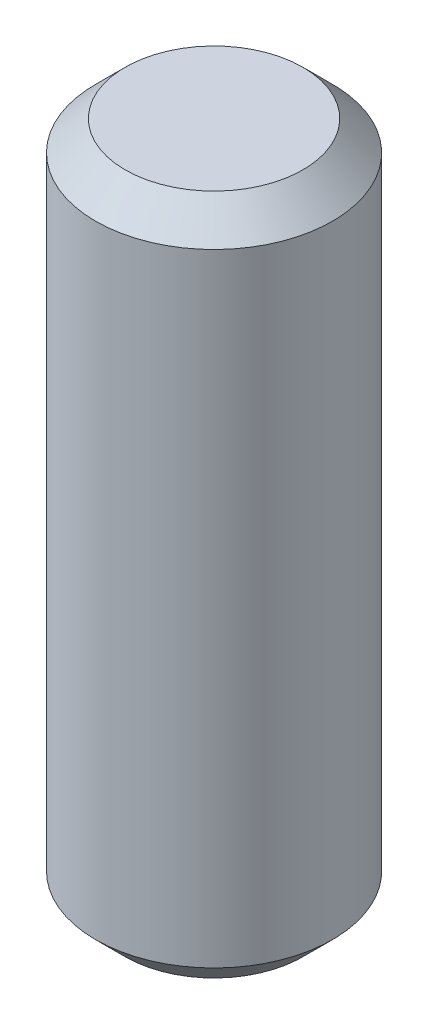
SolidWorks part; units mm, degrees
material "Plain Carbon Steel"
ref_plane "Front Plane" through (0, 0, 0) normal (0, 0, 1) x (1, 0, 0)
ref_plane "Top Plane" through (0, 0, 0) normal (0, 1, 0) x (1, 0, 0)
ref_plane "Right Plane" through (0, 0, 0) normal (1, 0, 0) x (0, 0, -1)
sketch "Pin Profile Ø4" plane through (0, 0, 0) normal (0, 1, 0) x (1, 0, 0)
  circle A0 centre (0, 0) radius 2
  dimension "D1" = 4
extrude "Pin Body Ø4x18" add sketch "Pin Profile Ø4" along normal blind 11.5
chamfer "End Chamfer A 0.5x45°" distance 0.5 angle 45 1 edges at (0, 11.5, 2)
chamfer "End Chamfer B 0.5x45°" distance 0.5 angle 45 1 edges at (0, 0, 2)
